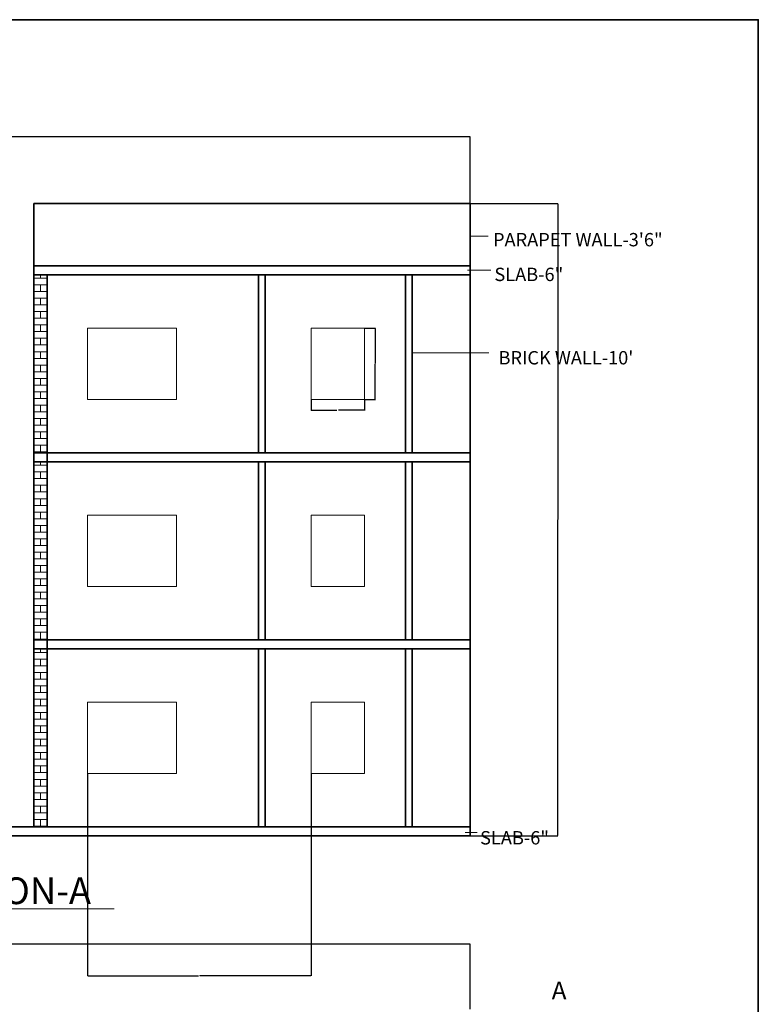
# Model space of a CAD drawing. Units: inches. Extents: x 2120 to 4013, y 1390 to 3019.
# Tile 59 of 59: x 3515 to 4013, y 2356 to 3019. Entities that reach past the tile are written whole.
import ezdxf

# ---------------------------------------------------------------- set-up
doc = ezdxf.new("R2010")
doc.units = ezdxf.units.IN
for name, color, linetype, lineweight in [('A-ANNO-DIMS', 2, 'Continuous', 18), ('A-ANNO-SYMB', 2, 'Continuous', 25), ('A-ANNO-TEXT', 7, 'Continuous', 18), ('A-ANNO-TTLB', 7, 'Continuous', 35), ('A-GLAZ', 4, 'Continuous', 18), ('A-SECT', 7, 'Continuous', 35), ('A-WALL-PATT', 252, 'Continuous', 13)]:
    doc.layers.add(name, color=color, linetype=linetype, lineweight=lineweight)
doc.styles.get("Standard").update_dxf_attribs({"font": 'arial.ttf'})
doc.dimstyles.get("Standard").update_dxf_attribs({"dimtxt": 0.18, "dimasz": 0.18, "dimexe": 0.18, "dimexo": 0.0625, "dimgap": 0.09, "dimtad": 0, "dimtih": 1, "dimtoh": 1, "dimdec": 4, "dimzin": 0, "dimdsep": 46, "dimtxsty": 'Standard', "dimcen": 0.09, "dimadec": 0, "dimazin": 0, "dimtfac": 1, "dimtdec": 4, "dimtofl": 0, "dimtmove": 0, "dimatfit": 3, "dimfxl": 1, "dimtolj": 1, "dimtzin": 0, "dimarcsym": 0})

# ---------------------------------------------------------------- blocks, each defined once
blk = doc.blocks.new('WIN-SECT-60IN')
for p, q in [((0, 48), (0, 0)), ((60, 48), (0, 48)), ((60, 48), (60, 0)), ((60, 0), (0, 0))]:
    blk.add_line(p, q)
blk = doc.blocks.new('WIN-SECT-36IN')
for p, q in [((0, 48), (0, 0)), ((36, 48), (0, 48)), ((36, 48), (36, 0)), ((36, 0), (0, 0))]:
    blk.add_line(p, q)
blk = doc.blocks.new('*D199')
at = {"layer": 'A-ANNO-DIMS', "color": 0, "lineweight": -2, "transparency": 16777216}
for p, q in [((3747.59, 2811.31), (3754.91, 2811.31)), ((3754.73, 2811.13), (3754.73, 2787.49)), ((3754.73, 2763.49), (3754.73, 2787.13)), ((3747.59, 2763.31), (3754.91, 2763.31))]:
    blk.add_line(p, q, dxfattribs=at)
at = {"layer": 'A-ANNO-DIMS', "color": 0, "transparency": 16777216}
for points in [[(3754.7, 2811.13), (3754.76, 2811.13), (3754.73, 2811.31)], [(3754.7, 2763.49), (3754.76, 2763.49), (3754.73, 2763.31)]]:
    blk.add_solid(points, dxfattribs=at)
at = {"layer": 'Defpoints', "color": 0, "transparency": 16777216}
for p in [(3747.53, 2811.31), (3754.73, 2811.31), (3747.53, 2763.31)]:
    blk.add_point(p, dxfattribs=at)
at = {"layer": 'A-ANNO-DIMS', "color": 0, "transparency": 16777216, "insert": (3754.73, 2787.31), "char_height": 0.18, "attachment_point": 5}
blk.add_mtext('\\A1;WINDOW 48 TYP.', dxfattribs=at)
blk = doc.blocks.new('*D200')
at = {"layer": 'A-ANNO-DIMS', "color": 0, "lineweight": -2, "transparency": 16777216}
for p, q in [((3711.53, 2763.25), (3711.53, 2755.93)), ((3747.53, 2763.25), (3747.53, 2755.93)), ((3711.71, 2756.11), (3729, 2756.11)), ((3747.35, 2756.11), (3730.06, 2756.11))]:
    blk.add_line(p, q, dxfattribs=at)
at = {"layer": 'A-ANNO-DIMS', "color": 0, "transparency": 16777216}
for points in [[(3711.71, 2756.14), (3711.71, 2756.08), (3711.53, 2756.11)], [(3747.35, 2756.14), (3747.35, 2756.08), (3747.53, 2756.11)]]:
    blk.add_solid(points, dxfattribs=at)
at = {"layer": 'Defpoints', "color": 0, "transparency": 16777216}
for p in [(3711.53, 2763.31), (3747.53, 2763.31), (3747.53, 2756.11)]:
    blk.add_point(p, dxfattribs=at)
at = {"layer": 'A-ANNO-DIMS', "color": 0, "transparency": 16777216, "insert": (3729.53, 2756.11), "char_height": 0.18, "attachment_point": 5}
blk.add_mtext('\\A1;36 TYP.', dxfattribs=at)
blk = doc.blocks.new('*D216')
at = {"layer": 'A-ANNO-DIMS', "color": 0, "lineweight": -2, "transparency": 16777216}
for p, q in [((3071.73, 2352.59), (3071.73, 2396.46)), ((3071.91, 2396.28), (3444.95, 2396.28)), ((3818.55, 2396.28), (3445.52, 2396.28)), ((3818.73, 2352.59), (3818.73, 2396.46))]:
    blk.add_line(p, q, dxfattribs=at)
at = {"layer": 'A-ANNO-DIMS', "color": 0, "transparency": 16777216}
for points in [[(3071.91, 2396.31), (3071.91, 2396.25), (3071.73, 2396.28)], [(3818.55, 2396.31), (3818.55, 2396.25), (3818.73, 2396.28)]]:
    blk.add_solid(points, dxfattribs=at)
at = {"layer": 'Defpoints', "color": 0, "transparency": 16777216}
for p in [(3818.73, 2396.28), (3071.73, 2352.53), (3818.73, 2352.53)]:
    blk.add_point(p, dxfattribs=at)
at = {"layer": 'A-ANNO-DIMS', "color": 0, "transparency": 16777216, "insert": (3445.23, 2396.28), "char_height": 0.18, "attachment_point": 5}
blk.add_mtext('\\A1;747', dxfattribs=at)
blk = doc.blocks.new('*D236')
at = {"layer": 'A-ANNO-DIMS', "color": 0, "lineweight": -2, "transparency": 16777216}
for p, q in [((3071.73, 2895.37), (3071.73, 2940.44)), ((3071.91, 2940.26), (3444.95, 2940.26)), ((3818.55, 2940.26), (3445.52, 2940.26)), ((3818.73, 2895.37), (3818.73, 2940.44))]:
    blk.add_line(p, q, dxfattribs=at)
at = {"layer": 'A-ANNO-DIMS', "color": 0, "transparency": 16777216}
for points in [[(3071.91, 2940.29), (3071.91, 2940.23), (3071.73, 2940.26)], [(3818.55, 2940.29), (3818.55, 2940.23), (3818.73, 2940.26)]]:
    blk.add_solid(points, dxfattribs=at)
at = {"layer": 'Defpoints', "color": 0, "transparency": 16777216}
for p in [(3818.73, 2940.26), (3071.73, 2895.31), (3818.73, 2895.31)]:
    blk.add_point(p, dxfattribs=at)
at = {"layer": 'A-ANNO-DIMS', "color": 0, "transparency": 16777216, "insert": (3445.23, 2940.26), "char_height": 0.18, "attachment_point": 5}
blk.add_mtext('\\A1;747', dxfattribs=at)
blk = doc.blocks.new('*D237')
at = {"layer": 'A-ANNO-DIMS', "color": 0, "lineweight": -2, "transparency": 16777216}
for p, q in [((3818.8, 2895.31), (3877.93, 2895.31)), ((3877.75, 2895.13), (3877.75, 2682.49)), ((3877.75, 2469.49), (3877.75, 2682.13)), ((3818.8, 2469.31), (3877.93, 2469.31))]:
    blk.add_line(p, q, dxfattribs=at)
at = {"layer": 'A-ANNO-DIMS', "color": 0, "transparency": 16777216}
for points in [[(3877.72, 2895.13), (3877.78, 2895.13), (3877.75, 2895.31)], [(3877.72, 2469.49), (3877.78, 2469.49), (3877.75, 2469.31)]]:
    blk.add_solid(points, dxfattribs=at)
at = {"layer": 'Defpoints', "color": 0, "transparency": 16777216}
for p in [(3818.73, 2895.31), (3877.75, 2895.31), (3818.73, 2469.31)]:
    blk.add_point(p, dxfattribs=at)
at = {"layer": 'A-ANNO-DIMS', "color": 0, "transparency": 16777216, "insert": (3877.75, 2682.31), "char_height": 0.18, "attachment_point": 5}
blk.add_mtext('\\A1;426', dxfattribs=at)
blk = doc.blocks.new('*D245')
at = {"layer": 'A-ANNO-DIMS', "color": 0, "lineweight": -2, "transparency": 16777216}
for p, q in [((3560.88, 2511.25), (3560.88, 2374.91)), ((3711.53, 2511.25), (3711.53, 2374.91)), ((3561.06, 2375.09), (3635.75, 2375.09)), ((3711.35, 2375.09), (3636.66, 2375.09))]:
    blk.add_line(p, q, dxfattribs=at)
at = {"layer": 'A-ANNO-DIMS', "color": 0, "transparency": 16777216}
for points in [[(3561.06, 2375.12), (3561.06, 2375.06), (3560.88, 2375.09)], [(3711.35, 2375.12), (3711.35, 2375.06), (3711.53, 2375.09)]]:
    blk.add_solid(points, dxfattribs=at)
at = {"layer": 'Defpoints', "color": 0, "transparency": 16777216}
for p in [(3560.88, 2511.31), (3711.53, 2511.31), (3711.53, 2375.09)]:
    blk.add_point(p, dxfattribs=at)
at = {"layer": 'A-ANNO-DIMS', "color": 0, "transparency": 16777216, "insert": (3636.2, 2375.09), "char_height": 0.18, "attachment_point": 5}
blk.add_mtext('\\A1;150.65', dxfattribs=at)

msp = doc.modelspace()

# ---------------------------------------------------------------- hatches: boundary and pattern name
at = {"layer": 'A-WALL-PATT'}
h = msp.add_hatch(dxfattribs=at)
h.set_pattern_fill('ANSI32', color=256)
h.paths.add_polyline_path([(2271.7331, 2343.531), (2283.3788, 2343.531), (2283.3788, 2348.031), (2283.3788, 2352.5306), (2262.7331, 2352.5306), (2262.7331, 2182.638), (2267.2331, 2182.638), (2271.7331, 2182.638), (2271.7331, 2219.031), (2391.7331, 2219.031), (2391.7331, 2214.189), (2393.9831, 2214.189), (2396.2331, 2214.189), (2396.2331, 2219.031), (2420.2331, 2219.031), (2420.2331, 2225.7535), (2417.2197, 2225.7535), (2415.7331, 2225.7535), (2415.7331, 2223.5306), (2271.7331, 2223.5306)])
h.paths.add_polyline_path([(2380.0942, 2352.5306), (2343.3788, 2352.5306), (2343.3788, 2343.531), (2363.2331, 2343.531), (2363.2331, 2288.8489), (2365.4831, 2288.8489), (2367.7331, 2288.8489), (2367.7331, 2343.531), (2380.0942, 2343.531)], flags=17)
h.paths.add_polyline_path([(2432.4339, 2352.5306), (2404.0943, 2352.5306), (2404.0943, 2343.531), (2415.7331, 2343.531), (2415.7331, 2264.0306), (2367.7331, 2264.0306), (2367.7331, 2266.4872), (2363.2331, 2266.4872), (2363.2331, 2259.531), (2367.7331, 2259.531), (2415.7331, 2259.531), (2415.7331, 2255.0658), (2420.2331, 2255.0658), (2420.2331, 2259.531), (2424.5717, 2259.531), (2424.5717, 2261.781), (2424.5717, 2264.0306), (2420.2331, 2264.0306), (2420.2331, 2343.531), (2432.4339, 2343.531)])
h.paths.add_polyline_path([(2508.9115, 2352.5306), (2456.4339, 2352.5306), (2456.4339, 2343.531), (2468.2331, 2343.531), (2468.2331, 2264.0306), (2448.0487, 2264.0306), (2448.0487, 2259.531), (2468.2331, 2259.531), (2468.2331, 2255.5496), (2472.7331, 2255.5496), (2472.7331, 2343.531), (2508.9115, 2343.531)])
h.paths.add_polyline_path([(2637.7331, 2352.5306), (2544.9116, 2352.5306), (2544.9116, 2343.531), (2589.7331, 2343.531), (2633.2331, 2343.531), (2637.7331, 2343.531)])
h.paths.add_polyline_path([(2594.2331, 2343.5306), (2589.7331, 2343.5306), (2589.7331, 2259.5306), (2589.7331, 2252.4915), (2591.9831, 2252.4915), (2594.2331, 2252.4915)])
h.paths.add_polyline_path([(2637.7331, 2223.5306), (2594.2331, 2223.5306), (2594.2331, 2230.1988), (2591.9831, 2230.1988), (2589.7331, 2230.1988), (2589.7331, 2223.5306), (2472.7331, 2223.5306), (2468.2331, 2223.5306), (2468.2331, 2219.031), (2628.7331, 2219.031), (2628.7331, 2138.031), (2637.7331, 2138.031)])
h.paths.add_polyline_path([(3822.6535, 2458.4402), (3874.9468, 2458.4402), (3874.9468, 2476.9866), (3822.6535, 2476.9866)], flags=9)
h.paths.add_polyline_path([(3834.6921, 2781.8174), (3935.9206, 2781.8174), (3935.9206, 2800.3638), (3834.6921, 2800.3638)], flags=9)
h.paths.add_polyline_path([(3832.2843, 2837.9683), (3884.5776, 2837.9683), (3884.5776, 2856.5146), (3832.2843, 2856.5146)], flags=9)
h.paths.add_polyline_path([(3830.9388, 2861.4782), (3956.8958, 2861.4782), (3956.8958, 2880.0245), (3830.9388, 2880.0245)], flags=9)
h.paths.add_polyline_path([(3870.6966, 2352.5752), (3887.9272, 2352.5752), (3887.9272, 2377.3037), (3870.6966, 2377.3037)], flags=9)
h.paths.add_polyline_path([(3289.2701, 2413.161), (3435.2223, 2413.161), (3435.2223, 2450.2538), (3289.2701, 2450.2538)], flags=9)
h.paths.add_polyline_path([(2487.6944, 2414.3601), (2637.8335, 2414.3601), (2637.8335, 2451.4528), (2487.6944, 2451.4528)], flags=9)
h.paths.add_polyline_path([(2567.3724, 1457.9199), (2815.296, 1457.9199), (2815.296, 1495.0127), (2567.3724, 1495.0127)], flags=9)
h.paths.add_polyline_path([(2655.3825, 2093.2363), (2685.9555, 2093.2363), (2685.9555, 2111.8937), (2655.3825, 2111.8937)], flags=9)
h.paths.add_polyline_path([(2543.9218, 1550.6671), (2587.8406, 1550.6671), (2587.8406, 1569.3244), (2543.9218, 1569.3244)], flags=9)
h.paths.add_polyline_path([(2905.1384, 1543.8113), (2949.0572, 1543.8113), (2949.0572, 1562.4686), (2905.1384, 1562.4686)], flags=9)
h.paths.add_polyline_path([(2736.4118, 1702.4736), (2784.2153, 1702.4736), (2784.2153, 1721.1309), (2736.4118, 1721.1309)], flags=9)
h.paths.add_polyline_path([(2912.8666, 1710.4168), (2951.707, 1710.4168), (2951.707, 1729.0741), (2912.8666, 1729.0741)], flags=9)
h.paths.add_polyline_path([(2923.5785, 1763.5038), (2959.7279, 1763.5038), (2959.7279, 1782.1611), (2923.5785, 1782.1611)], flags=9)
h.paths.add_polyline_path([(2925.2114, 1809.6137), (2967.1861, 1809.6137), (2967.1861, 1828.271), (2925.2114, 1828.271)], flags=9)
h.paths.add_polyline_path([(2996.2711, 1878.9003), (2996.2711, 1913.109), (2977.6138, 1913.109), (2977.6138, 1878.9003)], flags=9)
h.paths.add_polyline_path([(2883.0859, 1895.7192), (2927.1855, 1895.7192), (2927.1855, 1914.3766), (2883.0859, 1914.3766)], flags=9)
h.paths.add_polyline_path([(2787.3924, 1810.8013), (2841.0213, 1810.8013), (2841.0213, 1829.4587), (2787.3924, 1829.4587)], flags=9)
h.paths.add_polyline_path([(2775.6399, 2101.7395), (2829.2689, 2101.7395), (2829.2689, 2120.3968), (2775.6399, 2120.3968)], flags=9)
h.paths.add_polyline_path([(2913.0263, 2075.817), (2951.8667, 2075.817), (2951.8667, 2094.4744), (2913.0263, 2094.4744)], flags=9)
h.paths.add_polyline_path([(2929.966, 2133.3669), (2966.1154, 2133.3669), (2966.1154, 2152.0243), (2929.966, 2152.0243)], flags=9)
h.paths.add_polyline_path([(2932.7502, 2182.6088), (2968.8996, 2182.6088), (2968.8996, 2201.2662), (2932.7502, 2201.2662)], flags=9)
h.paths.add_polyline_path([(2996.0681, 2266.3173), (2996.0681, 2300.5261), (2977.4108, 2300.5261), (2977.4108, 2266.3173)], flags=9)
h.paths.add_polyline_path([(2885.1039, 2279.2186), (2929.2035, 2279.2186), (2929.2035, 2297.8759), (2885.1039, 2297.8759)], flags=9)
h.paths.add_polyline_path([(2735.7042, 2218.3197), (2783.5078, 2218.3197), (2783.5078, 2236.9771), (2735.7042, 2236.9771)], flags=9)
h.paths.add_polyline_path([(2635.6049, 2044.0085), (2648.9678, 2044.0085), (2648.9678, 2054.312), (2635.6049, 2054.312)], flags=9)
h.paths.add_polyline_path([(2714.0148, 1923.0473), (2727.3777, 1923.0473), (2727.3777, 1933.3508), (2714.0148, 1933.3508)], flags=9)
h.paths.add_polyline_path([(2709.0345, 1988.1628), (2722.3974, 1988.1628), (2722.3974, 1998.4663), (2709.0345, 1998.4663)], flags=9)
h.paths.add_polyline_path([(2592.8935, 1962.1763), (2606.2564, 1962.1763), (2606.2564, 1972.4799), (2592.8935, 1972.4799)], flags=9)
h.paths.add_polyline_path([(2618.3996, 1985.9724), (2644.1942, 1985.9724), (2644.1942, 1996.2759), (2618.3996, 1996.2759)], flags=9)
h.paths.add_polyline_path([(2601.279, 1920.5869), (2614.6419, 1920.5869), (2614.6419, 1930.8904), (2601.279, 1930.8904)], flags=9)
h.paths.add_polyline_path([(2692.3278, 1932.7645), (2704.5311, 1932.7645), (2704.5311, 1943.0681), (2692.3278, 1943.0681)], flags=9)
h.paths.add_polyline_path([(2311.122, 1672.7318), (2355.0408, 1672.7318), (2355.0408, 1691.3892), (2311.122, 1691.3892)], flags=9)
h.paths.add_polyline_path([(2456.2551, 1632.3198), (2492.4796, 1632.3198), (2492.4796, 1650.9772), (2456.2551, 1650.9772)], flags=9)
h.paths.add_polyline_path([(2401.0766, 1631.4793), (2437.301, 1631.4793), (2437.301, 1650.1367), (2401.0766, 1650.1367)], flags=9)
h.paths.add_polyline_path([(2546.7054, 1700.9235), (2594.509, 1700.9235), (2594.509, 1719.5809), (2546.7054, 1719.5809)], flags=9)
h.paths.add_polyline_path([(2445.4866, 1766.9937), (2497.5261, 1766.9937), (2497.5261, 1785.651), (2445.4866, 1785.651)], flags=9)
h.paths.add_polyline_path([(2287.9992, 1739.7675), (2326.8396, 1739.7675), (2326.8396, 1758.4248), (2287.9992, 1758.4248)], flags=9)
h.paths.add_polyline_path([(2458.5279, 1924.7607), (2510.5675, 1924.7607), (2510.5675, 1943.4181), (2458.5279, 1943.4181)], flags=9)
h.paths.add_polyline_path([(2309.2811, 1902.7642), (2345.4305, 1902.7642), (2345.4305, 1921.4215), (2309.2811, 1921.4215)], flags=9)
h.paths.add_polyline_path([(2490.7554, 2018.9392), (2530.7896, 2018.9392), (2530.7896, 2037.5965), (2490.7554, 2037.5965)], flags=9)
h.paths.add_polyline_path([(2402.143, 2024.7393), (2438.5414, 2024.7393), (2438.5414, 2043.3966), (2402.143, 2043.3966)], flags=9)
h.paths.add_polyline_path([(2287.856, 1931.7926), (2326.6964, 1931.7926), (2326.6964, 1950.4499), (2287.856, 1950.4499)], flags=9)
h.paths.add_polyline_path([(2281.7979, 2193.5771), (2320.6383, 2193.5771), (2320.6383, 2212.2344), (2281.7979, 2212.2344)], flags=25)
h.paths.add_polyline_path([(2484.0754, 2093.892), (2536.115, 2093.892), (2536.115, 2112.5494), (2484.0754, 2112.5494)], flags=9)
h.paths.add_polyline_path([(2624.7948, 2281.8639), (2624.7948, 2311.4137), (2606.1375, 2311.4137), (2606.1375, 2281.8639)], flags=9)
h.paths.add_polyline_path([(2507.5036, 2290.3639), (2541.934, 2290.3639), (2541.934, 2309.0212), (2507.5036, 2309.0212)], flags=9)
h.paths.add_polyline_path([(2423.1076, 2285.2202), (2459.332, 2285.2202), (2459.332, 2303.8776), (2423.1076, 2303.8776)], flags=9)
h.paths.add_polyline_path([(2374.5467, 2289.6272), (2410.7711, 2289.6272), (2410.7711, 2308.2846), (2374.5467, 2308.2846)], flags=25)
h.paths.add_polyline_path([(2277.4907, 2227.5651), (2316.3311, 2227.5651), (2316.3311, 2246.2224), (2277.4907, 2246.2224)], flags=25)
h.paths.add_polyline_path([(2655.3825, 2093.2367), (2685.9555, 2093.2367), (2685.9555, 2111.894), (2655.3825, 2111.894)], flags=9)
h.paths.add_polyline_path([(2543.9217, 1550.6674), (2587.8406, 1550.6674), (2587.8406, 1569.3247), (2543.9217, 1569.3247)], flags=9)
h.paths.add_polyline_path([(2905.1384, 1543.8116), (2949.0572, 1543.8116), (2949.0572, 1562.4689), (2905.1384, 1562.4689)], flags=9)
h.paths.add_polyline_path([(2736.4118, 1702.4739), (2784.2153, 1702.4739), (2784.2153, 1721.1312), (2736.4118, 1721.1312)], flags=9)
h.paths.add_polyline_path([(2912.8666, 1710.4171), (2951.707, 1710.4171), (2951.707, 1729.0744), (2912.8666, 1729.0744)], flags=9)
h.paths.add_polyline_path([(2923.5785, 1763.5041), (2959.7279, 1763.5041), (2959.7279, 1782.1614), (2923.5785, 1782.1614)], flags=9)
h.paths.add_polyline_path([(2925.2114, 1809.614), (2967.1861, 1809.614), (2967.1861, 1828.2713), (2925.2114, 1828.2713)], flags=9)
h.paths.add_polyline_path([(2996.2711, 1878.9006), (2996.2711, 1913.1094), (2977.6137, 1913.1094), (2977.6137, 1878.9006)], flags=9)
h.paths.add_polyline_path([(2883.0859, 1895.7195), (2927.1855, 1895.7195), (2927.1855, 1914.3769), (2883.0859, 1914.3769)], flags=9)
h.paths.add_polyline_path([(2787.3924, 1810.8016), (2841.0213, 1810.8016), (2841.0213, 1829.459), (2787.3924, 1829.459)], flags=9)
h.paths.add_polyline_path([(2775.6399, 2101.7398), (2829.2688, 2101.7398), (2829.2688, 2120.3971), (2775.6399, 2120.3971)], flags=9)
h.paths.add_polyline_path([(2913.0263, 2075.8173), (2951.8667, 2075.8173), (2951.8667, 2094.4747), (2913.0263, 2094.4747)], flags=9)
h.paths.add_polyline_path([(2929.966, 2133.3672), (2966.1154, 2133.3672), (2966.1154, 2152.0246), (2929.966, 2152.0246)], flags=9)
h.paths.add_polyline_path([(2932.7502, 2182.6091), (2968.8996, 2182.6091), (2968.8996, 2201.2665), (2932.7502, 2201.2665)], flags=9)
h.paths.add_polyline_path([(2996.0681, 2266.3176), (2996.0681, 2300.5264), (2977.4108, 2300.5264), (2977.4108, 2266.3176)], flags=9)
h.paths.add_polyline_path([(2885.1039, 2279.2189), (2929.2035, 2279.2189), (2929.2035, 2297.8762), (2885.1039, 2297.8762)], flags=9)
h.paths.add_polyline_path([(2735.7042, 2218.32), (2783.5078, 2218.32), (2783.5078, 2236.9774), (2735.7042, 2236.9774)], flags=9)
h.paths.add_polyline_path([(2635.6048, 2044.0088), (2648.9677, 2044.0088), (2648.9677, 2054.3123), (2635.6048, 2054.3123)], flags=9)
h.paths.add_polyline_path([(2714.0148, 1923.0476), (2727.3777, 1923.0476), (2727.3777, 1933.3511), (2714.0148, 1933.3511)], flags=9)
h.paths.add_polyline_path([(2709.0345, 1988.1631), (2722.3974, 1988.1631), (2722.3974, 1998.4666), (2709.0345, 1998.4666)], flags=9)
h.paths.add_polyline_path([(2592.8935, 1962.1766), (2606.2564, 1962.1766), (2606.2564, 1972.4802), (2592.8935, 1972.4802)], flags=9)
h.paths.add_polyline_path([(2618.3995, 1985.9727), (2644.1942, 1985.9727), (2644.1942, 1996.2762), (2618.3995, 1996.2762)], flags=9)
h.paths.add_polyline_path([(2601.279, 1920.5872), (2614.6419, 1920.5872), (2614.6419, 1930.8908), (2601.279, 1930.8908)], flags=9)
h.paths.add_polyline_path([(2692.3278, 1932.7648), (2704.5311, 1932.7648), (2704.5311, 1943.0684), (2692.3278, 1943.0684)], flags=9)
h.paths.add_polyline_path([(2311.122, 1672.7321), (2355.0408, 1672.7321), (2355.0408, 1691.3895), (2311.122, 1691.3895)], flags=9)
h.paths.add_polyline_path([(2456.2551, 1632.3201), (2492.4795, 1632.3201), (2492.4795, 1650.9775), (2456.2551, 1650.9775)], flags=9)
h.paths.add_polyline_path([(2401.0766, 1631.4796), (2437.301, 1631.4796), (2437.301, 1650.137), (2401.0766, 1650.137)], flags=9)
h.paths.add_polyline_path([(2546.7054, 1700.9238), (2594.509, 1700.9238), (2594.509, 1719.5812), (2546.7054, 1719.5812)], flags=9)
h.paths.add_polyline_path([(2445.4866, 1766.994), (2497.5261, 1766.994), (2497.5261, 1785.6513), (2445.4866, 1785.6513)], flags=9)
h.paths.add_polyline_path([(2287.9992, 1739.7678), (2326.8396, 1739.7678), (2326.8396, 1758.4251), (2287.9992, 1758.4251)], flags=9)
h.paths.add_polyline_path([(2458.5279, 1924.7611), (2510.5675, 1924.7611), (2510.5675, 1943.4184), (2458.5279, 1943.4184)], flags=9)
h.paths.add_polyline_path([(2309.2811, 1902.7645), (2345.4305, 1902.7645), (2345.4305, 1921.4218), (2309.2811, 1921.4218)], flags=9)
h.paths.add_polyline_path([(2490.7554, 2018.9395), (2530.7895, 2018.9395), (2530.7895, 2037.5968), (2490.7554, 2037.5968)], flags=9)
h.paths.add_polyline_path([(2402.143, 2024.7396), (2438.5413, 2024.7396), (2438.5413, 2043.3969), (2402.143, 2043.3969)], flags=9)
h.paths.add_polyline_path([(2287.856, 1931.7929), (2326.6964, 1931.7929), (2326.6964, 1950.4502), (2287.856, 1950.4502)], flags=9)
h.paths.add_polyline_path([(2281.7979, 2193.5774), (2320.6383, 2193.5774), (2320.6383, 2212.2347), (2281.7979, 2212.2347)], flags=25)
h.paths.add_polyline_path([(2484.0754, 2093.8924), (2536.115, 2093.8924), (2536.115, 2112.5497), (2484.0754, 2112.5497)], flags=9)
h.paths.add_polyline_path([(2624.7948, 2281.8642), (2624.7948, 2311.414), (2606.1374, 2311.414), (2606.1374, 2281.8642)], flags=9)
h.paths.add_polyline_path([(2507.5035, 2290.3642), (2541.934, 2290.3642), (2541.934, 2309.0215), (2507.5035, 2309.0215)], flags=9)
h.paths.add_polyline_path([(2423.1075, 2285.2205), (2459.332, 2285.2205), (2459.332, 2303.8779), (2423.1075, 2303.8779)], flags=9)
h.paths.add_polyline_path([(2374.5467, 2289.6275), (2410.7711, 2289.6275), (2410.7711, 2308.2849), (2374.5467, 2308.2849)], flags=25)
h.paths.add_polyline_path([(2277.4907, 2227.5654), (2316.3311, 2227.5654), (2316.3311, 2246.2227), (2277.4907, 2246.2227)], flags=25)
h = msp.add_hatch(dxfattribs=at)
h.set_pattern_fill('ANSI32', color=256)
h.paths.add_polyline_path([(2271.7331, 1980.389), (2262.7331, 1980.389), (2262.7331, 1912.8434), (2267.2331, 1912.8434), (2271.7331, 1912.8434), (2271.7331, 1922.531), (2351.2331, 1922.531), (2351.2331, 1901.4728), (2355.7331, 1901.4728), (2355.7331, 1922.531), (2357.9815, 1922.531), (2357.9815, 1926.5306), (2271.7331, 1926.5306)])
h.paths.add_polyline_path([(2589.2331, 1949.1622), (2584.7331, 1949.1622), (2580.2331, 1949.1622), (2580.2331, 1874.5306), (2355.7331, 1874.5306), (2355.7331, 1880.1922), (2351.2331, 1880.1922), (2351.2331, 1874.5306), (2271.7331, 1874.5306), (2271.7331, 1888.8431), (2262.7331, 1888.8431), (2262.7331, 1842.2909), (2267.2331, 1842.2909), (2271.7331, 1842.2909), (2271.7331, 1865.531), (2415.7331, 1865.531), (2415.7331, 1779.7286), (2420.2331, 1779.7286), (2420.2331, 1865.531), (2589.2331, 1865.531)])
h.paths.add_polyline_path([(2271.7331, 1782.2906), (2262.7331, 1782.2906), (2262.7331, 1711.4639), (2267.2331, 1711.4639), (2271.7331, 1711.4639), (2271.7331, 1738.031), (2420.2331, 1738.031), (2420.2331, 1742.531), (2420.2331, 1747.3376), (2417.9831, 1747.3376), (2415.7331, 1747.3376), (2415.7331, 1742.5306), (2271.7331, 1742.5306)])
h.paths.add_polyline_path([(2271.7331, 1627.031), (2362.3957, 1627.031), (2362.3957, 1629.281), (2362.3957, 1631.5306), (2271.7331, 1631.5306), (2271.7331, 1675.4636), (2262.7331, 1675.4636), (2262.7331, 1581.531), (2405.3032, 1581.531), (2405.3032, 1586.031), (2405.3032, 1590.5306), (2396.2331, 1590.5306), (2396.2331, 1691.4513), (2418.7206, 1691.4513), (2418.7206, 1695.951), (2396.2331, 1695.951), (2391.7331, 1695.951), (2391.7331, 1631.5306), (2386.7425, 1631.5306), (2386.7425, 1629.2806), (2386.7425, 1627.031), (2391.7331, 1627.031), (2391.7331, 1586.1709), (2271.7331, 1586.1709)])
h.paths.add_polyline_path([(2459.6703, 1590.5306), (2429.3032, 1590.5306), (2429.3032, 1581.531), (2459.6703, 1581.531), (2459.6703, 1586.031)])
h.paths.add_polyline_path([(2501.2331, 1590.531), (2501.2331, 1665.0195), (2498.9831, 1665.0195), (2496.7331, 1665.0195), (2496.7331, 1590.5306), (2483.8201, 1590.5306), (2483.8201, 1590.1579), (2483.6704, 1590.1579), (2483.6704, 1581.531), (2505.0196, 1581.531), (2505.0196, 1583.781), (2505.0196, 1586.0306), (2501.2331, 1586.0306)])
h.paths.add_polyline_path([(2544.1361, 1583.781), (2544.1361, 1586.0306), (2527.1368, 1586.0306), (2527.1368, 1583.7806), (2527.1368, 1581.531), (2544.1361, 1581.531)])
h.paths.add_polyline_path([(3822.6535, 2458.4402), (3874.9468, 2458.4402), (3874.9468, 2476.9866), (3822.6535, 2476.9866)], flags=9)
h.paths.add_polyline_path([(3834.6921, 2781.8174), (3935.9206, 2781.8174), (3935.9206, 2800.3638), (3834.6921, 2800.3638)], flags=9)
h.paths.add_polyline_path([(3832.2843, 2837.9683), (3884.5776, 2837.9683), (3884.5776, 2856.5146), (3832.2843, 2856.5146)], flags=9)
h.paths.add_polyline_path([(3830.9388, 2861.4782), (3956.8958, 2861.4782), (3956.8958, 2880.0245), (3830.9388, 2880.0245)], flags=9)
h.paths.add_polyline_path([(3870.6966, 2352.5752), (3887.9272, 2352.5752), (3887.9272, 2377.3037), (3870.6966, 2377.3037)], flags=9)
h.paths.add_polyline_path([(3289.2701, 2413.161), (3435.2223, 2413.161), (3435.2223, 2450.2538), (3289.2701, 2450.2538)], flags=9)
h.paths.add_polyline_path([(2487.6944, 2414.3601), (2637.8335, 2414.3601), (2637.8335, 2451.4528), (2487.6944, 2451.4528)], flags=9)
h.paths.add_polyline_path([(2567.3724, 1457.9199), (2815.296, 1457.9199), (2815.296, 1495.0127), (2567.3724, 1495.0127)], flags=9)
h.paths.add_polyline_path([(2655.3825, 2093.2363), (2685.9555, 2093.2363), (2685.9555, 2111.8937), (2655.3825, 2111.8937)], flags=9)
h.paths.add_polyline_path([(2543.9218, 1550.6671), (2587.8406, 1550.6671), (2587.8406, 1569.3244), (2543.9218, 1569.3244)], flags=9)
h.paths.add_polyline_path([(2905.1384, 1543.8113), (2949.0572, 1543.8113), (2949.0572, 1562.4686), (2905.1384, 1562.4686)], flags=9)
h.paths.add_polyline_path([(2736.4118, 1702.4736), (2784.2153, 1702.4736), (2784.2153, 1721.1309), (2736.4118, 1721.1309)], flags=9)
h.paths.add_polyline_path([(2912.8666, 1710.4168), (2951.707, 1710.4168), (2951.707, 1729.0741), (2912.8666, 1729.0741)], flags=9)
h.paths.add_polyline_path([(2923.5785, 1763.5038), (2959.7279, 1763.5038), (2959.7279, 1782.1611), (2923.5785, 1782.1611)], flags=9)
h.paths.add_polyline_path([(2925.2114, 1809.6137), (2967.1861, 1809.6137), (2967.1861, 1828.271), (2925.2114, 1828.271)], flags=9)
h.paths.add_polyline_path([(2996.2711, 1878.9003), (2996.2711, 1913.109), (2977.6138, 1913.109), (2977.6138, 1878.9003)], flags=9)
h.paths.add_polyline_path([(2883.0859, 1895.7192), (2927.1855, 1895.7192), (2927.1855, 1914.3766), (2883.0859, 1914.3766)], flags=9)
h.paths.add_polyline_path([(2787.3924, 1810.8013), (2841.0213, 1810.8013), (2841.0213, 1829.4587), (2787.3924, 1829.4587)], flags=9)
h.paths.add_polyline_path([(2775.6399, 2101.7395), (2829.2689, 2101.7395), (2829.2689, 2120.3968), (2775.6399, 2120.3968)], flags=9)
h.paths.add_polyline_path([(2913.0263, 2075.817), (2951.8667, 2075.817), (2951.8667, 2094.4744), (2913.0263, 2094.4744)], flags=9)
h.paths.add_polyline_path([(2929.966, 2133.3669), (2966.1154, 2133.3669), (2966.1154, 2152.0243), (2929.966, 2152.0243)], flags=9)
h.paths.add_polyline_path([(2932.7502, 2182.6088), (2968.8996, 2182.6088), (2968.8996, 2201.2662), (2932.7502, 2201.2662)], flags=9)
h.paths.add_polyline_path([(2996.0681, 2266.3173), (2996.0681, 2300.5261), (2977.4108, 2300.5261), (2977.4108, 2266.3173)], flags=9)
h.paths.add_polyline_path([(2885.1039, 2279.2186), (2929.2035, 2279.2186), (2929.2035, 2297.8759), (2885.1039, 2297.8759)], flags=9)
h.paths.add_polyline_path([(2735.7042, 2218.3197), (2783.5078, 2218.3197), (2783.5078, 2236.9771), (2735.7042, 2236.9771)], flags=9)
h.paths.add_polyline_path([(2635.6049, 2044.0085), (2648.9678, 2044.0085), (2648.9678, 2054.312), (2635.6049, 2054.312)], flags=9)
h.paths.add_polyline_path([(2714.0148, 1923.0473), (2727.3777, 1923.0473), (2727.3777, 1933.3508), (2714.0148, 1933.3508)], flags=9)
h.paths.add_polyline_path([(2709.0345, 1988.1628), (2722.3974, 1988.1628), (2722.3974, 1998.4663), (2709.0345, 1998.4663)], flags=9)
h.paths.add_polyline_path([(2592.8935, 1962.1763), (2606.2564, 1962.1763), (2606.2564, 1972.4799), (2592.8935, 1972.4799)], flags=9)
h.paths.add_polyline_path([(2618.3996, 1985.9724), (2644.1942, 1985.9724), (2644.1942, 1996.2759), (2618.3996, 1996.2759)], flags=9)
h.paths.add_polyline_path([(2601.279, 1920.5869), (2614.6419, 1920.5869), (2614.6419, 1930.8904), (2601.279, 1930.8904)], flags=9)
h.paths.add_polyline_path([(2692.3278, 1932.7645), (2704.5311, 1932.7645), (2704.5311, 1943.0681), (2692.3278, 1943.0681)], flags=9)
h.paths.add_polyline_path([(2311.122, 1672.7318), (2355.0408, 1672.7318), (2355.0408, 1691.3892), (2311.122, 1691.3892)], flags=25)
h.paths.add_polyline_path([(2456.2551, 1632.3198), (2492.4796, 1632.3198), (2492.4796, 1650.9772), (2456.2551, 1650.9772)], flags=9)
h.paths.add_polyline_path([(2401.0766, 1631.4793), (2437.301, 1631.4793), (2437.301, 1650.1367), (2401.0766, 1650.1367)], flags=9)
h.paths.add_polyline_path([(2546.7054, 1700.9235), (2594.509, 1700.9235), (2594.509, 1719.5809), (2546.7054, 1719.5809)], flags=9)
h.paths.add_polyline_path([(2445.4866, 1766.9937), (2497.5261, 1766.9937), (2497.5261, 1785.651), (2445.4866, 1785.651)], flags=9)
h.paths.add_polyline_path([(2287.9992, 1739.7675), (2326.8396, 1739.7675), (2326.8396, 1758.4248), (2287.9992, 1758.4248)], flags=24)
h.paths.add_polyline_path([(2458.5279, 1924.7607), (2510.5675, 1924.7607), (2510.5675, 1943.4181), (2458.5279, 1943.4181)], flags=25)
h.paths.add_polyline_path([(2309.2811, 1902.7642), (2345.4305, 1902.7642), (2345.4305, 1921.4215), (2309.2811, 1921.4215)], flags=25)
h.paths.add_polyline_path([(2490.7554, 2018.9392), (2530.7896, 2018.9392), (2530.7896, 2037.5965), (2490.7554, 2037.5965)], flags=9)
h.paths.add_polyline_path([(2402.143, 2024.7393), (2438.5414, 2024.7393), (2438.5414, 2043.3966), (2402.143, 2043.3966)], flags=9)
h.paths.add_polyline_path([(2287.856, 1931.7926), (2326.6964, 1931.7926), (2326.6964, 1950.4499), (2287.856, 1950.4499)], flags=25)
h.paths.add_polyline_path([(2281.7979, 2193.5771), (2320.6383, 2193.5771), (2320.6383, 2212.2344), (2281.7979, 2212.2344)], flags=9)
h.paths.add_polyline_path([(2484.0754, 2093.892), (2536.115, 2093.892), (2536.115, 2112.5494), (2484.0754, 2112.5494)], flags=9)
h.paths.add_polyline_path([(2624.7948, 2281.8639), (2624.7948, 2311.4137), (2606.1375, 2311.4137), (2606.1375, 2281.8639)], flags=9)
h.paths.add_polyline_path([(2507.5036, 2290.3639), (2541.934, 2290.3639), (2541.934, 2309.0212), (2507.5036, 2309.0212)], flags=9)
h.paths.add_polyline_path([(2423.1076, 2285.2202), (2459.332, 2285.2202), (2459.332, 2303.8776), (2423.1076, 2303.8776)], flags=9)
h.paths.add_polyline_path([(2374.5467, 2289.6272), (2410.7711, 2289.6272), (2410.7711, 2308.2846), (2374.5467, 2308.2846)], flags=9)
h.paths.add_polyline_path([(2277.4907, 2227.5651), (2316.3311, 2227.5651), (2316.3311, 2246.2224), (2277.4907, 2246.2224)], flags=9)
h.paths.add_polyline_path([(2655.3825, 2093.2367), (2685.9555, 2093.2367), (2685.9555, 2111.894), (2655.3825, 2111.894)], flags=9)
h.paths.add_polyline_path([(2543.9217, 1550.6674), (2587.8406, 1550.6674), (2587.8406, 1569.3247), (2543.9217, 1569.3247)], flags=9)
h.paths.add_polyline_path([(2905.1384, 1543.8116), (2949.0572, 1543.8116), (2949.0572, 1562.4689), (2905.1384, 1562.4689)], flags=9)
h.paths.add_polyline_path([(2736.4118, 1702.4739), (2784.2153, 1702.4739), (2784.2153, 1721.1312), (2736.4118, 1721.1312)], flags=9)
h.paths.add_polyline_path([(2912.8666, 1710.4171), (2951.707, 1710.4171), (2951.707, 1729.0744), (2912.8666, 1729.0744)], flags=9)
h.paths.add_polyline_path([(2923.5785, 1763.5041), (2959.7279, 1763.5041), (2959.7279, 1782.1614), (2923.5785, 1782.1614)], flags=9)
h.paths.add_polyline_path([(2925.2114, 1809.614), (2967.1861, 1809.614), (2967.1861, 1828.2713), (2925.2114, 1828.2713)], flags=9)
h.paths.add_polyline_path([(2996.2711, 1878.9006), (2996.2711, 1913.1094), (2977.6137, 1913.1094), (2977.6137, 1878.9006)], flags=9)
h.paths.add_polyline_path([(2883.0859, 1895.7195), (2927.1855, 1895.7195), (2927.1855, 1914.3769), (2883.0859, 1914.3769)], flags=9)
h.paths.add_polyline_path([(2787.3924, 1810.8016), (2841.0213, 1810.8016), (2841.0213, 1829.459), (2787.3924, 1829.459)], flags=9)
h.paths.add_polyline_path([(2775.6399, 2101.7398), (2829.2688, 2101.7398), (2829.2688, 2120.3971), (2775.6399, 2120.3971)], flags=9)
h.paths.add_polyline_path([(2913.0263, 2075.8173), (2951.8667, 2075.8173), (2951.8667, 2094.4747), (2913.0263, 2094.4747)], flags=9)
h.paths.add_polyline_path([(2929.966, 2133.3672), (2966.1154, 2133.3672), (2966.1154, 2152.0246), (2929.966, 2152.0246)], flags=9)
h.paths.add_polyline_path([(2932.7502, 2182.6091), (2968.8996, 2182.6091), (2968.8996, 2201.2665), (2932.7502, 2201.2665)], flags=9)
h.paths.add_polyline_path([(2996.0681, 2266.3176), (2996.0681, 2300.5264), (2977.4108, 2300.5264), (2977.4108, 2266.3176)], flags=9)
h.paths.add_polyline_path([(2885.1039, 2279.2189), (2929.2035, 2279.2189), (2929.2035, 2297.8762), (2885.1039, 2297.8762)], flags=9)
h.paths.add_polyline_path([(2735.7042, 2218.32), (2783.5078, 2218.32), (2783.5078, 2236.9774), (2735.7042, 2236.9774)], flags=9)
h.paths.add_polyline_path([(2635.6048, 2044.0088), (2648.9677, 2044.0088), (2648.9677, 2054.3123), (2635.6048, 2054.3123)], flags=9)
h.paths.add_polyline_path([(2714.0148, 1923.0476), (2727.3777, 1923.0476), (2727.3777, 1933.3511), (2714.0148, 1933.3511)], flags=9)
h.paths.add_polyline_path([(2709.0345, 1988.1631), (2722.3974, 1988.1631), (2722.3974, 1998.4666), (2709.0345, 1998.4666)], flags=9)
h.paths.add_polyline_path([(2592.8935, 1962.1766), (2606.2564, 1962.1766), (2606.2564, 1972.4802), (2592.8935, 1972.4802)], flags=9)
h.paths.add_polyline_path([(2618.3995, 1985.9727), (2644.1942, 1985.9727), (2644.1942, 1996.2762), (2618.3995, 1996.2762)], flags=9)
h.paths.add_polyline_path([(2601.279, 1920.5872), (2614.6419, 1920.5872), (2614.6419, 1930.8908), (2601.279, 1930.8908)], flags=9)
h.paths.add_polyline_path([(2692.3278, 1932.7648), (2704.5311, 1932.7648), (2704.5311, 1943.0684), (2692.3278, 1943.0684)], flags=9)
h.paths.add_polyline_path([(2311.122, 1672.7321), (2355.0408, 1672.7321), (2355.0408, 1691.3895), (2311.122, 1691.3895)], flags=25)
h.paths.add_polyline_path([(2456.2551, 1632.3201), (2492.4795, 1632.3201), (2492.4795, 1650.9775), (2456.2551, 1650.9775)], flags=9)
h.paths.add_polyline_path([(2401.0766, 1631.4796), (2437.301, 1631.4796), (2437.301, 1650.137), (2401.0766, 1650.137)], flags=9)
h.paths.add_polyline_path([(2546.7054, 1700.9238), (2594.509, 1700.9238), (2594.509, 1719.5812), (2546.7054, 1719.5812)], flags=9)
h.paths.add_polyline_path([(2445.4866, 1766.994), (2497.5261, 1766.994), (2497.5261, 1785.6513), (2445.4866, 1785.6513)], flags=9)
h.paths.add_polyline_path([(2287.9992, 1739.7678), (2326.8396, 1739.7678), (2326.8396, 1758.4251), (2287.9992, 1758.4251)], flags=24)
h.paths.add_polyline_path([(2458.5279, 1924.7611), (2510.5675, 1924.7611), (2510.5675, 1943.4184), (2458.5279, 1943.4184)], flags=25)
h.paths.add_polyline_path([(2309.2811, 1902.7645), (2345.4305, 1902.7645), (2345.4305, 1921.4218), (2309.2811, 1921.4218)], flags=25)
h.paths.add_polyline_path([(2490.7554, 2018.9395), (2530.7895, 2018.9395), (2530.7895, 2037.5968), (2490.7554, 2037.5968)], flags=9)
h.paths.add_polyline_path([(2402.143, 2024.7396), (2438.5413, 2024.7396), (2438.5413, 2043.3969), (2402.143, 2043.3969)], flags=9)
h.paths.add_polyline_path([(2287.856, 1931.7929), (2326.6964, 1931.7929), (2326.6964, 1950.4502), (2287.856, 1950.4502)], flags=25)
h.paths.add_polyline_path([(2281.7979, 2193.5774), (2320.6383, 2193.5774), (2320.6383, 2212.2347), (2281.7979, 2212.2347)], flags=9)
h.paths.add_polyline_path([(2484.0754, 2093.8924), (2536.115, 2093.8924), (2536.115, 2112.5497), (2484.0754, 2112.5497)], flags=9)
h.paths.add_polyline_path([(2624.7948, 2281.8642), (2624.7948, 2311.414), (2606.1374, 2311.414), (2606.1374, 2281.8642)], flags=9)
h.paths.add_polyline_path([(2507.5035, 2290.3642), (2541.934, 2290.3642), (2541.934, 2309.0215), (2507.5035, 2309.0215)], flags=9)
h.paths.add_polyline_path([(2423.1075, 2285.2205), (2459.332, 2285.2205), (2459.332, 2303.8779), (2423.1075, 2303.8779)], flags=9)
h.paths.add_polyline_path([(2374.5467, 2289.6275), (2410.7711, 2289.6275), (2410.7711, 2308.2849), (2374.5467, 2308.2849)], flags=9)
h.paths.add_polyline_path([(2277.4907, 2227.5654), (2316.3311, 2227.5654), (2316.3311, 2246.2227), (2277.4907, 2246.2227)], flags=9)
h = msp.add_hatch(dxfattribs=at)
h.set_pattern_fill('BRICK', color=256, scale=0.70891, style=0)
h.paths.add_polyline_path([(3524.7347, 2727.3118), (3533.7347, 2727.3118), (3533.7347, 2847.3118), (3524.7347, 2847.3118)])
h = msp.add_hatch(dxfattribs=at)
h.set_pattern_fill('BRICK', color=256, scale=0.70891, style=0)
h.paths.add_polyline_path([(3524.7347, 2601.3118), (3533.7347, 2601.3118), (3533.7347, 2721.3118), (3524.7347, 2721.3118)])
h = msp.add_hatch(dxfattribs=at)
h.set_pattern_fill('BRICK', color=256, scale=0.70891, style=0)
h.paths.add_polyline_path([(3524.7347, 2475.3118), (3533.7347, 2475.3118), (3533.7347, 2595.3118), (3524.7347, 2595.3118)])

# ---------------------------------------------------------------- linework, layer by layer
at = {"layer": 'A-ANNO-TEXT'}
for p, q in [((3818.7347, 2873.3684), (3830.9971, 2873.3684)), ((3816.9489, 2850.3742), (3832.8039, 2850.3742)), ((3779.7347, 2794.6171), (3831.4345, 2794.6171)), ((3815.3767, 2471.4757), (3823.4438, 2471.4757)), ((3578.9077, 2420.0416), (3434.336, 2420.0416))]:
    msp.add_line(p, q, dxfattribs=at)
at = {"layer": 'A-ANNO-TTLB'}
msp.add_lwpolyline([(2120.4581, 3019.1237), (4012.9334, 3019.1237), (4012.9334, 1390.2222), (2120.4581, 1390.2222)], close=True, dxfattribs=at)
at = {"layer": 'A-SECT'}
for p, q in [((3524.7347, 2895.3118), (3524.7347, 2727.3118)), ((3818.7347, 2895.3118), (3524.7347, 2895.3118)), ((3818.7347, 2895.3118), (3818.7347, 2709.3118)), ((3818.7347, 2853.3118), (3524.7347, 2853.3118)), ((3818.7347, 2847.3118), (3524.7347, 2847.3118)), ((3533.7347, 2847.3118), (3533.7347, 2727.3118)), ((3676.2347, 2847.3118), (3676.2347, 2727.3118)), ((3680.7347, 2847.3118), (3680.7347, 2727.3118)), ((3775.2347, 2847.3118), (3775.2347, 2727.3118)), ((3779.7347, 2847.3118), (3779.7347, 2727.3118)), ((3818.7347, 2769.3118), (3818.7347, 2583.3118)), ((3524.7347, 2727.3118), (3524.7347, 2595.3118)), ((3818.7347, 2727.3118), (3524.7347, 2727.3118)), ((3533.7347, 2727.3118), (3533.7347, 2595.3118)), ((3818.7347, 2721.3118), (3524.7347, 2721.3118)), ((3676.2347, 2721.3118), (3676.2347, 2601.3118)), ((3680.7347, 2721.3118), (3680.7347, 2601.3118)), ((3775.2347, 2721.3118), (3775.2347, 2601.3118)), ((3779.7347, 2721.3118), (3779.7347, 2601.3118)), ((3818.7347, 2643.3118), (3818.7347, 2469.3118)), ((3818.7347, 2601.3118), (3524.7347, 2601.3118)), ((3524.7347, 2595.3118), (3524.7347, 2475.3118)), ((3818.7347, 2595.3118), (3524.7347, 2595.3118)), ((3533.7347, 2595.3118), (3533.7347, 2475.3118)), ((3676.2347, 2595.3118), (3676.2347, 2475.3118)), ((3680.7347, 2595.3118), (3680.7347, 2475.3118)), ((3775.2347, 2595.3118), (3775.2347, 2475.3118)), ((3779.7347, 2595.3118), (3779.7347, 2475.3118)), ((3818.7347, 2475.3118), (3071.7347, 2475.3118)), ((3071.7347, 2469.3118), (3818.7347, 2469.3118))]:
    msp.add_line(p, q, dxfattribs=at)

# ---------------------------------------------------------------- block references
at = {"layer": 'A-GLAZ', "rotation": 180}
for p in [(3620.877, 2811.3118), (3620.877, 2685.3118), (3620.877, 2559.3118)]:
    msp.add_blockref('WIN-SECT-60IN', p, dxfattribs=at)
at = {"layer": 'A-GLAZ'}
for p in [(3711.5315, 2763.3118), (3711.5315, 2637.3118), (3711.5315, 2511.3118)]:
    msp.add_blockref('WIN-SECT-36IN', p, dxfattribs=at)

# ---------------------------------------------------------------- texts
at = {"layer": 'A-ANNO-SYMB', "insert": (3873.7212, 2371.1277), "char_height": 12, "attachment_point": 1}
msp.add_mtext_dynamic_manual_height_columns('A', width=58.697611, gutter_width=12.5, heights=[0], dxfattribs=at)
at = {"layer": 'A-ANNO-TEXT', "attachment_point": 1}
for s, width, insert, char_height in [('PARAPET WALL-3\'6"', 283.931717, (3834.1588, 2875.4294), 9), ('SLAB-6"', 80.107266, (3835.0991, 2852.0361), 9), ("BRICK WALL-10'", 201.879175, (3837.8629, 2795.8852), 9), ('SLAB-6"', 48.480737, (3825.4683, 2472.5081), 9), ('SECTION-A', 601.378558, (3437.2118, 2441.309), 18)]:
    msp.add_mtext_dynamic_manual_height_columns(s, width=width, gutter_width=12.5, heights=[0], dxfattribs=dict(at, insert=insert, char_height=char_height))

# ---------------------------------------------------------------- dimensions: what is measured, and where the dimension line sits
at = {"layer": 'A-ANNO-DIMS'}
for base, p1, p2, override, picture, middle in [((3818.7347, 2940.2618), (3071.7347, 2895.3118), (3818.7347, 2895.3118), {"dimdec": 0, "dimlfac": 1, "dimrnd": 0, "dimzin": 0, "dimdsep": 46, "dimlunit": 2}, '*D236', (3445.2347, 2940.2618)), ((3711.5315, 2375.0916), (3560.877, 2511.3118), (3711.5315, 2511.3118), {"dimdec": 2, "dimlfac": 1, "dimrnd": 0, "dimzin": 0, "dimdsep": 46, "dimlunit": 2}, '*D245', (3636.2043, 2375.0916)), ((3818.7347, 2396.281), (3071.7347, 2352.531), (3818.7347, 2352.531), {"dimdec": 0, "dimlfac": 1, "dimrnd": 0, "dimzin": 0, "dimdsep": 46, "dimlunit": 2}, '*D216', (3445.2347, 2396.281))]:
    dim = msp.add_linear_dim(base=base, p1=p1, p2=p2, dimstyle='Standard', override=override, dxfattribs=at)
    dim.commit()
    dim.dimension.update_dxf_attribs({"geometry": picture, "text_midpoint": middle})
dim = msp.add_linear_dim(base=(3877.7539, 2895.3118), p1=(3818.7347, 2469.3118), p2=(3818.7347, 2895.3118), angle=90, dimstyle='Standard', override={"dimdec": 0, "dimlfac": 1, "dimrnd": 0, "dimzin": 0, "dimdsep": 46, "dimlunit": 2}, dxfattribs=at)
dim.commit()
dim.dimension.update_dxf_attribs({"geometry": '*D237', "text_midpoint": (3877.7539, 2682.3118)})
dim = msp.add_linear_dim(base=(3754.7315, 2811.3118), p1=(3747.5315, 2763.3118), p2=(3747.5315, 2811.3118), angle=90, text='WINDOW <> TYP.', dimstyle='Standard', override={"dimdec": 0, "dimlfac": 1, "dimrnd": 0, "dimzin": 0, "dimdsep": 46, "dimlunit": 2}, dxfattribs=at)
dim.commit()
dim.dimension.update_dxf_attribs({"geometry": '*D199', "text_midpoint": (3754.7315, 2787.3118)})
dim = msp.add_linear_dim(base=(3747.5315, 2756.1118), p1=(3711.5315, 2763.3118), p2=(3747.5315, 2763.3118), text='<> TYP.', dimstyle='Standard', override={"dimdec": 0, "dimlfac": 1, "dimrnd": 0, "dimzin": 0, "dimdsep": 46, "dimlunit": 2}, dxfattribs=at)
dim.commit()
dim.dimension.update_dxf_attribs({"geometry": '*D200', "text_midpoint": (3729.5315, 2756.1118)})

doc.saveas('drawing.dxf')
